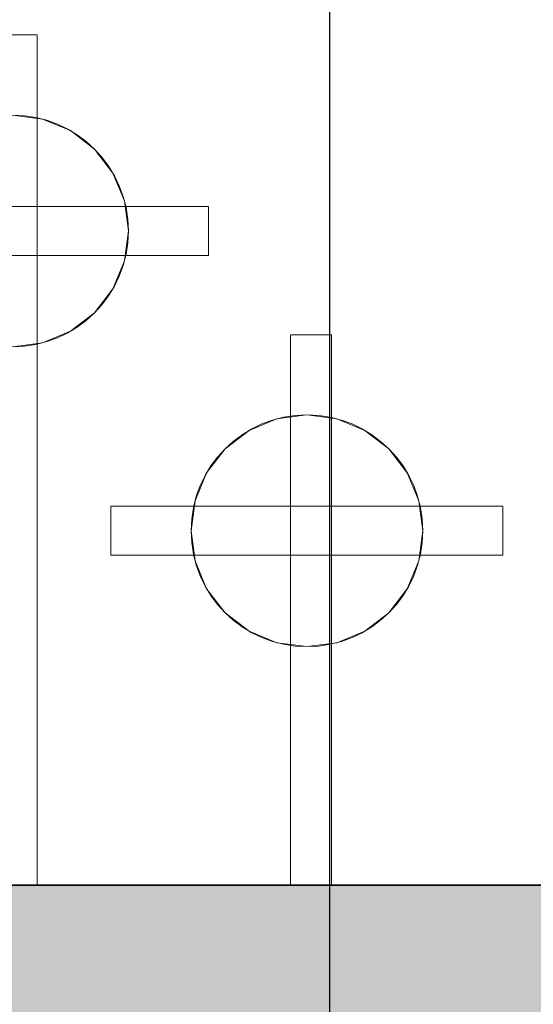
# Model space of a CAD drawing. Units: inches. Extents: x 2696 to 3240, y 1564 to 2310.
# Tile 31 of 76: x 3146.244 to 3150.171, y 1698.791 to 1706.319. Entities that reach past the tile are written whole.
import ezdxf

# ---------------------------------------------------------------- set-up
doc = ezdxf.new("R2010")
doc.units = ezdxf.units.IN
for name, color, linetype, lineweight in [('A-ANNO-DIMS', 3, 'Continuous', 18), ('A-FLOR-FIXT', 8, 'Continuous', 18), ('A-FURN', 251, 'Continuous', 13), ('A-WALL', 7, 'Continuous', 35), ('A-WALL-PATT', 9, 'Continuous', 13)]:
    doc.layers.add(name, color=color, linetype=linetype, lineweight=lineweight)
doc.layers.add('FURNITURE', color=250, linetype='Continuous')
doc.styles.add('TIMES NEW', font='times.ttf')
doc.dimstyles.new('Siddhuu', dxfattribs={"dimtxt": 6, "dimasz": 2.5, "dimexe": 1.25, "dimexo": 0.625, "dimtad": 1, "dimdec": 1, "dimlunit": 4, "dimtxsty": 'TIMES NEW', "dimcen": 2.5, "dimclrd": 256, "dimclre": 1, "dimclrt": 7, "dimadec": 0, "dimazin": 0, "dimtfac": 1, "dimtdec": 1, "dimtmove": 0, "dimatfit": 3, "dimfxl": 1, "dimtolj": 1, "dimlwd": -1, "dimarcsym": 0})

# ---------------------------------------------------------------- blocks, each defined once
blk = doc.blocks.new('A$C1af1f523')
at = {"layer": 'A-FURN'}
for p, q in [((-5.1906, 1.6871), (-5.1901, -1.3115)), ((-5.1906, 1.6871, 0.5), (-5.1901, -1.3115, 0.5)), ((-4.8156, 1.6871), (-4.8151, -1.3115)), ((-4.8156, 1.6871, 0.5), (-4.8151, -1.3115, 0.5)), ((-6.5015, 0.3114), (-6.5015, 0)), ((-6.5015, 0.3114, 0.5), (-6.5015, 0, 0.5)), ((0, 0), (-6.5015, 0)), ((0, 0, 0.5), (-6.5015, 0, 0.5)), ((-6.5015, 0), (-6.5015, 0, 0.5)), ((-6.5015, 0), (-6.5015, -0.0011)), ((-6.5015, 0, 0.5), (-6.5015, -0.0011, 0.5)), ((-6.5015, -0.0011), (-6.5015, -0.0011, 0.5)), ((-5.8585, -0.0418), (-5.8585, -0.0418, 0.5)), ((-4.1468, -0.0418), (-4.1468, -0.0418, 0.5)), ((-5.77, -0.2555), (-5.77, -0.2555, 0.5)), ((-4.2353, -0.2555), (-4.2353, -0.2555, 0.5)), ((-5.6292, -0.439), (-5.6292, -0.439, 0.5)), ((-4.3761, -0.439), (-4.3761, -0.439, 0.5)), ((-5.4457, -0.5798), (-5.4457, -0.5798, 0.5)), ((-4.5596, -0.5798), (-4.5596, -0.5798, 0.5)), ((-2.898, -0.5642), (-2.898, -3.5628)), ((-2.898, -0.5642, 0.5), (-2.898, -3.5628, 0.5)), ((-2.898, -0.5642), (-2.898, -0.5642, 0.5)), ((-2.523, -0.5642), (-2.898, -0.5642)), ((-2.523, -0.5642, 0.5), (-2.898, -0.5642, 0.5)), ((-2.523, -0.5642), (-2.523, -3.5628)), ((-2.523, -0.5642, 0.5), (-2.523, -3.5628, 0.5)), ((-2.523, -0.5642), (-2.523, -0.5642, 0.5)), ((-5.232, -0.6683), (-5.232, -0.6683, 0.5)), ((-4.7733, -0.6683), (-4.7733, -0.6683, 0.5)), ((-5.0026, -0.6985), (-5.0026, -0.6985, 0.5)), ((-2.7105, -1.1778), (-2.7105, -1.1778, 0.5)), ((-2.9398, -1.208), (-2.9398, -1.208, 0.5)), ((-2.4812, -1.208), (-2.4812, -1.208, 0.5)), ((-5.1901, -1.3115), (-5.1901, -1.3115, 0.5)), ((-4.8151, -1.3115), (-5.1878, -1.3115)), ((-4.8151, -1.3115, 0.5), (-5.1878, -1.3115, 0.5)), ((-5.1878, -1.3115), (-5.1878, -1.3115, 0.5)), ((-4.8151, -1.3115), (-4.8151, -1.3115, 0.5)), ((-3.1535, -1.2965), (-3.1535, -1.2965, 0.5)), ((-2.2675, -1.2965), (-2.2675, -1.2965, 0.5)), ((-3.337, -1.4373), (-3.337, -1.4373, 0.5)), ((-2.084, -1.4373), (-2.084, -1.4373, 0.5)), ((-3.4778, -1.6208), (-3.4778, -1.6208, 0.5)), ((-1.9432, -1.6208), (-1.9432, -1.6208, 0.5)), ((-3.5664, -1.8345), (-3.5664, -1.8345, 0.5)), ((-1.8547, -1.8345), (-1.8547, -1.8345, 0.5)), ((0, -1.9388), (-4.2094, -1.9388)), ((0, -1.9388, 0.5), (-4.2094, -1.9388, 0.5)), ((-4.2094, -1.9388), (-4.2094, -1.9388, 0.5)), ((-4.2094, -1.9399), (-4.2094, -2.2513)), ((-4.2094, -1.9399, 0.5), (-4.2094, -2.2513, 0.5)), ((-4.2094, -1.9399), (-4.2094, -1.9399, 0.5)), ((-3.5965, -2.0638), (-3.5965, -2.0638, 0.5)), ((-1.8245, -2.0638), (-1.8245, -2.0638, 0.5)), ((0, -2.2513), (-4.2094, -2.2513)), ((0, -2.2513, 0.5), (-4.2094, -2.2513, 0.5)), ((-4.2094, -2.2513), (-4.2094, -2.2513, 0.5)), ((-4.2094, -2.2513), (-4.2094, -2.2524)), ((-4.2094, -2.2513, 0.5), (-4.2094, -2.2524, 0.5)), ((-4.2094, -2.2524), (-4.2094, -2.2524, 0.5)), ((-3.5664, -2.2931), (-3.5664, -2.2931, 0.5)), ((-1.8547, -2.2931), (-1.8547, -2.2931, 0.5)), ((-3.4778, -2.5068), (-3.4778, -2.5068, 0.5)), ((-1.9432, -2.5068), (-1.9432, -2.5068, 0.5)), ((-3.337, -2.6903), (-3.337, -2.6903, 0.5)), ((-2.084, -2.6903), (-2.084, -2.6903, 0.5)), ((-3.1535, -2.8311), (-3.1535, -2.8311, 0.5)), ((-2.2675, -2.8311), (-2.2675, -2.8311, 0.5)), ((-2.9398, -2.9196), (-2.9398, -2.9196, 0.5)), ((-2.4812, -2.9196), (-2.4812, -2.9196, 0.5)), ((-2.7105, -2.9498), (-2.7105, -2.9498, 0.5)), ((-2.898, -3.5628), (-2.898, -3.5628, 0.5)), ((-2.523, -3.5628), (-2.8956, -3.5628)), ((-2.523, -3.5628, 0.5), (-2.8956, -3.5628, 0.5)), ((-2.8956, -3.5628), (-2.8956, -3.5628, 0.5)), ((-2.523, -3.5628), (-2.523, -3.5628, 0.5))]:
    blk.add_line(p, q, dxfattribs=at)
for centre in [(-5.0026, 0.1875), (-5.0026, 0.1875, 0.5), (-2.7105, -2.0638), (-2.7105, -2.0638, 0.5)]:
    blk.add_circle(centre, 0.886, dxfattribs=at)
at = {"layer": 'FURNITURE'}
for p, q in [((0, 0), (0, 0, 0.5)), ((0, -1.9388), (0, -1.9388, 0.5)), ((0, -2.2513), (0, -2.2513, 0.5))]:
    blk.add_line(p, q, dxfattribs=at)
at = {"layer": 'A-FURN'}
mesh = blk.add_polyface(dxfattribs=at)
corners = [(-5.1901, -1.3115, 0.5), (-5.1906, 1.6871), (-5.1901, -1.3115), (-5.1906, 1.6871, 0.5)]
mesh.append_faces([[corners[k] for k in face] for face in [(2, 1, 0), (3, 0, 1)]], dxfattribs={"vtx1": -1})
mesh = blk.add_polyface(dxfattribs=at)
corners = [(-4.8151, -1.3115, 0.5), (-4.8156, 1.6871), (-4.8151, -1.3115), (-4.8156, 1.6871, 0.5)]
mesh.append_faces([[corners[k] for k in face] for face in [(2, 1, 0), (3, 0, 1)]], dxfattribs={"vtx1": -1})
mesh = blk.add_polyface(dxfattribs=at)
corners = [(-6.5015, -0.0011, 0.5), (-6.5015, 0), (-6.5015, -0.0011), (-6.5015, 0.3114), (-6.5015, 0.3114, 0.5), (-6.5015, 0, 0.5)]
mesh.append_faces([[corners[k] for k in face] for face in [(3, 0, 1), (4, 0, 3)]], dxfattribs={"vtx0": -1, "vtx1": -1})
mesh.append_faces([[corners[k] for k in face] for face in [(2, 1, 0), (5, 0, 4)]], dxfattribs={"vtx1": -1})
mesh = blk.add_polyface(dxfattribs=at)
corners = [(-5.8887, 0.1875, 0.5), (-5.8585, -0.0418), (-5.8887, 0.1875), (-5.8585, -0.0418, 0.5)]
mesh.append_faces([[corners[k] for k in face] for face in [(2, 1, 0), (3, 0, 1)]], dxfattribs={"vtx1": -1})
mesh = blk.add_polyface(dxfattribs=at)
corners = [(-4.1468, -0.0418, 0.5), (-4.1166, 0.1875), (-4.1468, -0.0418), (-4.1166, 0.1875, 0.5)]
mesh.append_faces([[corners[k] for k in face] for face in [(2, 1, 0), (3, 0, 1)]], dxfattribs={"vtx1": -1})
mesh = blk.add_polyface(dxfattribs=at)
corners = [(0, 0, 0.5), (-6.5015, 0), (-6.5015, 0, 0.5), (0, 0)]
mesh.append_faces([[corners[k] for k in face] for face in [(2, 1, 0), (3, 0, 1)]], dxfattribs={"vtx1": -1})
mesh = blk.add_polyface(dxfattribs=at)
corners = [(-5.8585, -0.0418, 0.5), (-5.77, -0.2555), (-5.8585, -0.0418), (-5.77, -0.2555, 0.5)]
mesh.append_faces([[corners[k] for k in face] for face in [(2, 1, 0), (3, 0, 1)]], dxfattribs={"vtx1": -1})
mesh = blk.add_polyface(dxfattribs=at)
corners = [(-4.2353, -0.2555, 0.5), (-4.1468, -0.0418), (-4.2353, -0.2555), (-4.1468, -0.0418, 0.5)]
mesh.append_faces([[corners[k] for k in face] for face in [(2, 1, 0), (3, 0, 1)]], dxfattribs={"vtx1": -1})
mesh = blk.add_polyface(dxfattribs=at)
corners = [(-5.77, -0.2555, 0.5), (-5.6292, -0.439), (-5.77, -0.2555), (-5.6292, -0.439, 0.5)]
mesh.append_faces([[corners[k] for k in face] for face in [(2, 1, 0), (3, 0, 1)]], dxfattribs={"vtx1": -1})
mesh = blk.add_polyface(dxfattribs=at)
corners = [(-4.3761, -0.439, 0.5), (-4.2353, -0.2555), (-4.3761, -0.439), (-4.2353, -0.2555, 0.5)]
mesh.append_faces([[corners[k] for k in face] for face in [(2, 1, 0), (3, 0, 1)]], dxfattribs={"vtx1": -1})
mesh = blk.add_polyface(dxfattribs=at)
corners = [(-5.4457, -0.5798, 0.5), (-5.6292, -0.439), (-5.6292, -0.439, 0.5), (-5.4457, -0.5798)]
mesh.append_faces([[corners[k] for k in face] for face in [(2, 1, 0), (3, 0, 1)]], dxfattribs={"vtx1": -1})
mesh = blk.add_polyface(dxfattribs=at)
corners = [(-4.3761, -0.439, 0.5), (-4.5596, -0.5798), (-4.5596, -0.5798, 0.5), (-4.3761, -0.439)]
mesh.append_faces([[corners[k] for k in face] for face in [(2, 1, 0), (3, 0, 1)]], dxfattribs={"vtx1": -1})
mesh = blk.add_polyface(dxfattribs=at)
corners = [(-5.232, -0.6683, 0.5), (-5.4457, -0.5798), (-5.4457, -0.5798, 0.5), (-5.232, -0.6683)]
mesh.append_faces([[corners[k] for k in face] for face in [(2, 1, 0), (3, 0, 1)]], dxfattribs={"vtx1": -1})
mesh = blk.add_polyface(dxfattribs=at)
corners = [(-4.5596, -0.5798, 0.5), (-4.7733, -0.6683), (-4.7733, -0.6683, 0.5), (-4.5596, -0.5798)]
mesh.append_faces([[corners[k] for k in face] for face in [(2, 1, 0), (3, 0, 1)]], dxfattribs={"vtx1": -1})
mesh = blk.add_polyface(dxfattribs=at)
corners = [(-2.898, -3.5628, 0.5), (-2.898, -0.5642), (-2.898, -3.5628), (-2.898, -0.5642, 0.5)]
mesh.append_faces([[corners[k] for k in face] for face in [(2, 1, 0), (3, 0, 1)]], dxfattribs={"vtx1": -1})
mesh = blk.add_polyface(dxfattribs=at)
corners = [(-2.523, -0.5642, 0.5), (-2.898, -0.5642), (-2.898, -0.5642, 0.5), (-2.523, -0.5642)]
mesh.append_faces([[corners[k] for k in face] for face in [(2, 1, 0), (3, 0, 1)]], dxfattribs={"vtx1": -1})
mesh = blk.add_polyface(dxfattribs=at)
corners = [(-2.523, -3.5628, 0.5), (-2.523, -0.5642), (-2.523, -3.5628), (-2.523, -0.5642, 0.5)]
mesh.append_faces([[corners[k] for k in face] for face in [(2, 1, 0), (3, 0, 1)]], dxfattribs={"vtx1": -1})
mesh = blk.add_polyface(dxfattribs=at)
corners = [(-5.0026, -0.6985, 0.5), (-5.232, -0.6683), (-5.232, -0.6683, 0.5), (-5.0026, -0.6985)]
mesh.append_faces([[corners[k] for k in face] for face in [(2, 1, 0), (3, 0, 1)]], dxfattribs={"vtx1": -1})
mesh = blk.add_polyface(dxfattribs=at)
corners = [(-4.7733, -0.6683, 0.5), (-5.0026, -0.6985), (-5.0026, -0.6985, 0.5), (-4.7733, -0.6683)]
mesh.append_faces([[corners[k] for k in face] for face in [(2, 1, 0), (3, 0, 1)]], dxfattribs={"vtx1": -1})
mesh = blk.add_polyface(dxfattribs=at)
corners = [(-2.7105, -1.1778), (-2.9398, -1.208, 0.5), (-2.9398, -1.208), (-2.7105, -1.1778, 0.5)]
mesh.append_faces([[corners[k] for k in face] for face in [(2, 1, 0), (3, 0, 1)]], dxfattribs={"vtx1": -1})
mesh = blk.add_polyface(dxfattribs=at)
corners = [(-2.4812, -1.208), (-2.7105, -1.1778, 0.5), (-2.7105, -1.1778), (-2.4812, -1.208, 0.5)]
mesh.append_faces([[corners[k] for k in face] for face in [(2, 1, 0), (3, 0, 1)]], dxfattribs={"vtx1": -1})
mesh = blk.add_polyface(dxfattribs=at)
corners = [(-2.9398, -1.208), (-3.1535, -1.2965, 0.5), (-3.1535, -1.2965), (-2.9398, -1.208, 0.5)]
mesh.append_faces([[corners[k] for k in face] for face in [(2, 1, 0), (3, 0, 1)]], dxfattribs={"vtx1": -1})
mesh = blk.add_polyface(dxfattribs=at)
corners = [(-2.2675, -1.2965), (-2.4812, -1.208, 0.5), (-2.4812, -1.208), (-2.2675, -1.2965, 0.5)]
mesh.append_faces([[corners[k] for k in face] for face in [(2, 1, 0), (3, 0, 1)]], dxfattribs={"vtx1": -1})
mesh = blk.add_polyface(dxfattribs=at)
corners = [(-4.8151, -1.3115, 0.5), (-5.1878, -1.3115), (-5.1878, -1.3115, 0.5), (-4.8151, -1.3115)]
mesh.append_faces([[corners[k] for k in face] for face in [(2, 1, 0), (3, 0, 1)]], dxfattribs={"vtx1": -1})
mesh = blk.add_polyface(dxfattribs=at)
corners = [(-3.1535, -1.2965), (-3.337, -1.4373, 0.5), (-3.337, -1.4373), (-3.1535, -1.2965, 0.5)]
mesh.append_faces([[corners[k] for k in face] for face in [(2, 1, 0), (3, 0, 1)]], dxfattribs={"vtx1": -1})
mesh = blk.add_polyface(dxfattribs=at)
corners = [(-2.084, -1.4373), (-2.2675, -1.2965, 0.5), (-2.2675, -1.2965), (-2.084, -1.4373, 0.5)]
mesh.append_faces([[corners[k] for k in face] for face in [(2, 1, 0), (3, 0, 1)]], dxfattribs={"vtx1": -1})
mesh = blk.add_polyface(dxfattribs=at)
corners = [(-3.337, -1.4373, 0.5), (-3.4778, -1.6208), (-3.337, -1.4373), (-3.4778, -1.6208, 0.5)]
mesh.append_faces([[corners[k] for k in face] for face in [(2, 1, 0), (3, 0, 1)]], dxfattribs={"vtx1": -1})
mesh = blk.add_polyface(dxfattribs=at)
corners = [(-1.9432, -1.6208, 0.5), (-2.084, -1.4373), (-1.9432, -1.6208), (-2.084, -1.4373, 0.5)]
mesh.append_faces([[corners[k] for k in face] for face in [(2, 1, 0), (3, 0, 1)]], dxfattribs={"vtx1": -1})
mesh = blk.add_polyface(dxfattribs=at)
corners = [(-3.4778, -1.6208, 0.5), (-3.5664, -1.8345), (-3.4778, -1.6208), (-3.5664, -1.8345, 0.5)]
mesh.append_faces([[corners[k] for k in face] for face in [(2, 1, 0), (3, 0, 1)]], dxfattribs={"vtx1": -1})
mesh = blk.add_polyface(dxfattribs=at)
corners = [(-1.8547, -1.8345, 0.5), (-1.9432, -1.6208), (-1.8547, -1.8345), (-1.9432, -1.6208, 0.5)]
mesh.append_faces([[corners[k] for k in face] for face in [(2, 1, 0), (3, 0, 1)]], dxfattribs={"vtx1": -1})
mesh = blk.add_polyface(dxfattribs=at)
corners = [(-3.5664, -1.8345, 0.5), (-3.5965, -2.0638), (-3.5664, -1.8345), (-3.5965, -2.0638, 0.5)]
mesh.append_faces([[corners[k] for k in face] for face in [(2, 1, 0), (3, 0, 1)]], dxfattribs={"vtx1": -1})
mesh = blk.add_polyface(dxfattribs=at)
corners = [(-1.8245, -2.0638, 0.5), (-1.8547, -1.8345), (-1.8245, -2.0638), (-1.8547, -1.8345, 0.5)]
mesh.append_faces([[corners[k] for k in face] for face in [(2, 1, 0), (3, 0, 1)]], dxfattribs={"vtx1": -1})
mesh = blk.add_polyface(dxfattribs=at)
corners = [(0, -1.9388, 0.5), (-4.2094, -1.9388), (-4.2094, -1.9388, 0.5), (0, -1.9388)]
mesh.append_faces([[corners[k] for k in face] for face in [(2, 1, 0), (3, 0, 1)]], dxfattribs={"vtx1": -1})
mesh = blk.add_polyface(dxfattribs=at)
corners = [(-4.2094, -2.2524, 0.5), (-4.2094, -2.2513), (-4.2094, -2.2524), (-4.2094, -1.9399), (-4.2094, -1.9399, 0.5), (-4.2094, -2.2513, 0.5)]
mesh.append_faces([[corners[k] for k in face] for face in [(3, 0, 1), (4, 0, 3)]], dxfattribs={"vtx0": -1, "vtx1": -1})
mesh.append_faces([[corners[k] for k in face] for face in [(2, 1, 0), (5, 0, 4)]], dxfattribs={"vtx1": -1})
mesh = blk.add_polyface(dxfattribs=at)
corners = [(-3.5965, -2.0638, 0.5), (-3.5664, -2.2931), (-3.5965, -2.0638), (-3.5664, -2.2931, 0.5)]
mesh.append_faces([[corners[k] for k in face] for face in [(2, 1, 0), (3, 0, 1)]], dxfattribs={"vtx1": -1})
mesh = blk.add_polyface(dxfattribs=at)
corners = [(-1.8547, -2.2931, 0.5), (-1.8245, -2.0638), (-1.8547, -2.2931), (-1.8245, -2.0638, 0.5)]
mesh.append_faces([[corners[k] for k in face] for face in [(2, 1, 0), (3, 0, 1)]], dxfattribs={"vtx1": -1})
mesh = blk.add_polyface(dxfattribs=at)
corners = [(0, -2.2513, 0.5), (-4.2094, -2.2513), (-4.2094, -2.2513, 0.5), (0, -2.2513)]
mesh.append_faces([[corners[k] for k in face] for face in [(2, 1, 0), (3, 0, 1)]], dxfattribs={"vtx1": -1})
mesh = blk.add_polyface(dxfattribs=at)
corners = [(-3.5664, -2.2931, 0.5), (-3.4778, -2.5068), (-3.5664, -2.2931), (-3.4778, -2.5068, 0.5)]
mesh.append_faces([[corners[k] for k in face] for face in [(2, 1, 0), (3, 0, 1)]], dxfattribs={"vtx1": -1})
mesh = blk.add_polyface(dxfattribs=at)
corners = [(-1.9432, -2.5068, 0.5), (-1.8547, -2.2931), (-1.9432, -2.5068), (-1.8547, -2.2931, 0.5)]
mesh.append_faces([[corners[k] for k in face] for face in [(2, 1, 0), (3, 0, 1)]], dxfattribs={"vtx1": -1})
mesh = blk.add_polyface(dxfattribs=at)
corners = [(-3.4778, -2.5068, 0.5), (-3.337, -2.6903), (-3.4778, -2.5068), (-3.337, -2.6903, 0.5)]
mesh.append_faces([[corners[k] for k in face] for face in [(2, 1, 0), (3, 0, 1)]], dxfattribs={"vtx1": -1})
mesh = blk.add_polyface(dxfattribs=at)
corners = [(-2.084, -2.6903, 0.5), (-1.9432, -2.5068), (-2.084, -2.6903), (-1.9432, -2.5068, 0.5)]
mesh.append_faces([[corners[k] for k in face] for face in [(2, 1, 0), (3, 0, 1)]], dxfattribs={"vtx1": -1})
mesh = blk.add_polyface(dxfattribs=at)
corners = [(-3.1535, -2.8311, 0.5), (-3.337, -2.6903), (-3.337, -2.6903, 0.5), (-3.1535, -2.8311)]
mesh.append_faces([[corners[k] for k in face] for face in [(2, 1, 0), (3, 0, 1)]], dxfattribs={"vtx1": -1})
mesh = blk.add_polyface(dxfattribs=at)
corners = [(-2.084, -2.6903, 0.5), (-2.2675, -2.8311), (-2.2675, -2.8311, 0.5), (-2.084, -2.6903)]
mesh.append_faces([[corners[k] for k in face] for face in [(2, 1, 0), (3, 0, 1)]], dxfattribs={"vtx1": -1})
mesh = blk.add_polyface(dxfattribs=at)
corners = [(-2.9398, -2.9196, 0.5), (-3.1535, -2.8311), (-3.1535, -2.8311, 0.5), (-2.9398, -2.9196)]
mesh.append_faces([[corners[k] for k in face] for face in [(2, 1, 0), (3, 0, 1)]], dxfattribs={"vtx1": -1})
mesh = blk.add_polyface(dxfattribs=at)
corners = [(-2.2675, -2.8311, 0.5), (-2.4812, -2.9196), (-2.4812, -2.9196, 0.5), (-2.2675, -2.8311)]
mesh.append_faces([[corners[k] for k in face] for face in [(2, 1, 0), (3, 0, 1)]], dxfattribs={"vtx1": -1})
mesh = blk.add_polyface(dxfattribs=at)
corners = [(-2.7105, -2.9498, 0.5), (-2.9398, -2.9196), (-2.9398, -2.9196, 0.5), (-2.7105, -2.9498)]
mesh.append_faces([[corners[k] for k in face] for face in [(2, 1, 0), (3, 0, 1)]], dxfattribs={"vtx1": -1})
mesh = blk.add_polyface(dxfattribs=at)
corners = [(-2.4812, -2.9196, 0.5), (-2.7105, -2.9498), (-2.7105, -2.9498, 0.5), (-2.4812, -2.9196)]
mesh.append_faces([[corners[k] for k in face] for face in [(2, 1, 0), (3, 0, 1)]], dxfattribs={"vtx1": -1})
mesh = blk.add_polyface(dxfattribs=at)
corners = [(-2.523, -3.5628, 0.5), (-2.8956, -3.5628), (-2.8956, -3.5628, 0.5), (-2.523, -3.5628)]
mesh.append_faces([[corners[k] for k in face] for face in [(2, 1, 0), (3, 0, 1)]], dxfattribs={"vtx1": -1})
blk = doc.blocks.new('*D51')
at = {"layer": 'A-ANNO-DIMS', "color": 1, "lineweight": -2, "transparency": 16777216}
for p, q in [((3016.6114, 1979.5761), (3016.6114, 1568.9511)), ((3148.6114, 1979.5761), (3148.6114, 1568.9511))]:
    blk.add_line(p, q, dxfattribs=at)
at = {"layer": 'A-ANNO-DIMS', "transparency": 16777216}
blk.add_line((3019.1114, 1570.2011), (3146.1114, 1570.2011), dxfattribs=at)
for points in [[(3019.1114, 1570.6178), (3019.1114, 1569.7844), (3016.6114, 1570.2011)], [(3146.1114, 1570.6178), (3146.1114, 1569.7844), (3148.6114, 1570.2011)]]:
    blk.add_solid(points, dxfattribs=at)
at = {"layer": 'Defpoints', "color": 0, "transparency": 16777216}
for p in [(3016.6114, 1980.2011), (3148.6114, 1980.2011), (3148.6114, 1570.2011)]:
    blk.add_point(p, dxfattribs=at)
at = {"layer": 'A-ANNO-DIMS', "color": 7, "transparency": 16777216, "insert": (3082.6114, 1573.878), "char_height": 6, "attachment_point": 5, "style": 'TIMES NEW'}
blk.add_mtext('\\A1;11\'-0"', dxfattribs=at)
blk = doc.blocks.new('*D52')
at = {"layer": 'A-ANNO-DIMS', "color": 1, "lineweight": -2, "transparency": 16777216}
for p, q in [((3148.6114, 1979.5761), (3148.6114, 1568.9511)), ((3190.6114, 1979.5761), (3190.6114, 1568.9511))]:
    blk.add_line(p, q, dxfattribs=at)
at = {"layer": 'A-ANNO-DIMS', "transparency": 16777216}
blk.add_line((3151.1114, 1570.2011), (3188.1114, 1570.2011), dxfattribs=at)
for points in [[(3151.1114, 1570.6178), (3151.1114, 1569.7844), (3148.6114, 1570.2011)], [(3188.1114, 1570.6178), (3188.1114, 1569.7844), (3190.6114, 1570.2011)]]:
    blk.add_solid(points, dxfattribs=at)
at = {"layer": 'Defpoints', "color": 0, "transparency": 16777216}
for p in [(3148.6114, 1980.2011), (3190.6114, 1980.2011), (3190.6114, 1570.2011)]:
    blk.add_point(p, dxfattribs=at)
at = {"layer": 'A-ANNO-DIMS', "color": 7, "transparency": 16777216, "insert": (3169.6114, 1573.878), "char_height": 6, "attachment_point": 5, "style": 'TIMES NEW'}
blk.add_mtext('\\A1;3\'-6"', dxfattribs=at)
blk = doc.blocks.new('*D56')
at = {"layer": 'A-ANNO-DIMS', "color": 1, "lineweight": -2, "transparency": 16777216}
for p, q in [((2966.3338, 1884.2011), (3235.8614, 1884.2011)), ((2966.3338, 1665.2011), (3235.8614, 1665.2011))]:
    blk.add_line(p, q, dxfattribs=at)
at = {"layer": 'A-ANNO-DIMS', "transparency": 16777216}
blk.add_line((3234.6114, 1667.7011), (3234.6114, 1881.7011), dxfattribs=at)
for points in [[(3234.1947, 1881.7011), (3235.0281, 1881.7011), (3234.6114, 1884.2011)], [(3234.1947, 1667.7011), (3235.0281, 1667.7011), (3234.6114, 1665.2011)]]:
    blk.add_solid(points, dxfattribs=at)
at = {"layer": 'Defpoints', "color": 0, "transparency": 16777216}
for p in [(2965.7088, 1884.2011), (3234.6114, 1884.2011), (2965.7088, 1665.2011)]:
    blk.add_point(p, dxfattribs=at)
at = {"layer": 'A-ANNO-DIMS', "color": 7, "transparency": 16777216, "insert": (3230.9345, 1774.7011), "char_height": 6, "attachment_point": 5, "rotation": 90, "style": 'TIMES NEW'}
blk.add_mtext('\\A1;18\'-3"', dxfattribs=at)

msp = doc.modelspace()

# ---------------------------------------------------------------- hatches: boundary and pattern name
at = {"layer": 'A-WALL-PATT', "transparency": 33554556}
h = msp.add_hatch(color=256, dxfattribs=at)
h.dxf.hatch_style = 1
h.paths.add_polyline_path([(2879.1114, 2253.2011), (2905.9101, 2253.2011), (2905.9101, 2262.2011), (2841.889, 2262.2011), (2841.889, 2253.2011), (2870.1114, 2253.2011), (2870.1114, 2176.6011), (2965.7088, 2176.6011), (2965.7088, 2206.7011), (2973.5828, 2206.7011), (2973.5828, 2215.7011), (2965.7088, 2215.7011), (2965.7088, 2262.2011), (2929.9101, 2262.2011), (2929.9101, 2253.2011), (2956.7088, 2253.2011), (2956.7088, 2185.6011), (2879.1114, 2185.6011)])
h.paths.add_polyline_path([(2782.8338, 2262.2011), (2745.6114, 2262.2011), (2745.6114, 2228.7287), (2754.6114, 2228.7287), (2754.6114, 2253.2011), (2782.8338, 2253.2011)])
h.paths.add_polyline_path([(2754.6114, 2136.2011), (2965.7088, 2136.2011), (2965.7088, 2145.2011), (2879.1114, 2145.2011), (2879.1114, 2147.0735), (2877.3397, 2147.0735), (2870.1114, 2147.0735), (2870.1114, 2145.2011), (2754.6114, 2145.2011), (2754.6114, 2169.6735), (2745.6114, 2169.6735), (2745.6114, 2000.2011), (2754.6114, 2000.2011), (2754.6114, 2019.2011), (2849.0828, 2019.2011), (2849.0828, 2023.7011), (2841.2088, 2023.7011), (2841.2088, 2051.8271), (2836.7088, 2051.8271), (2836.7088, 2023.7011), (2754.6114, 2023.7011), (2754.6114, 2091.2011), (2836.7088, 2091.2011), (2836.7088, 2087.8271), (2841.2088, 2087.8271), (2841.2088, 2095.7011), (2754.6114, 2095.7011)])
h.paths.add_polyline_path([(2965.7088, 2136.2011), (2956.7088, 2136.2011), (2956.7088, 2023.7011), (2885.0828, 2023.7011), (2885.0828, 2019.2011), (2956.7088, 2019.2011), (2956.7088, 1950.5751), (2965.7088, 1950.5751), (2965.7088, 1980.2011), (2973.5828, 1980.2011), (2973.5828, 1989.2011), (2965.7088, 1989.2011)])
h.paths.add_polyline_path([(2754.6114, 1906.7011), (2880.2088, 1906.7011), (2884.7088, 1906.7011), (2956.7088, 1906.7011), (2956.7088, 1792.7011), (2944.7088, 1792.7011), (2944.7088, 1783.7011), (2956.7088, 1783.7011), (2956.7088, 1740.2011), (2884.7088, 1740.2011), (2884.7088, 1783.7011), (2896.7088, 1783.7011), (2896.7088, 1792.7011), (2884.7088, 1792.7011), (2884.7088, 1846.7011), (2880.2088, 1846.7011), (2880.2088, 1740.2011), (2754.6114, 1740.2011), (2754.6114, 1777.2011), (2745.6114, 1777.2011), (2745.6114, 1692.7011), (2754.6114, 1692.7011), (2754.6114, 1731.2011), (2956.7088, 1731.2011), (2956.7088, 1723.3271), (2965.7088, 1723.3271), (2965.7088, 1884.2011), (2973.5828, 1884.2011), (2973.5828, 1893.2011), (2965.7088, 1893.2011), (2965.7088, 1914.5751), (2956.7088, 1914.5751), (2956.7088, 1911.2011), (2754.6114, 1911.2011), (2754.6114, 1930.2011), (2745.6114, 1930.2011), (2745.6114, 1817.2011), (2754.6114, 1817.2011), (2754.6114, 1854.2011), (2826.6114, 1854.2011), (2826.6114, 1868.8271), (2822.1114, 1868.8271), (2822.1114, 1858.7011), (2754.6114, 1858.7011)])
h.paths.add_polyline_path([(2965.7088, 1656.2011), (3008.2374, 1656.2011), (3008.2374, 1665.2011), (2965.7088, 1665.2011), (2965.7088, 1693.3271), (2956.7088, 1693.3271), (2956.7088, 1686.2011), (2934.5828, 1686.2011), (2934.5828, 1681.7011), (2956.7088, 1681.7011), (2956.7088, 1614.2011), (2896.7088, 1614.2011), (2896.7088, 1681.7011), (2904.5828, 1681.7011), (2904.5828, 1686.2011), (2892.2088, 1686.2011), (2892.2088, 1614.2011), (2858.4101, 1614.2011), (2858.4101, 1605.2011), (2965.7088, 1605.2011)])
h.paths.add_polyline_path([(2788.4101, 1614.2011), (2754.6114, 1614.2011), (2754.6114, 1652.7011), (2745.6114, 1652.7011), (2745.6114, 1605.2011), (2788.4101, 1605.2011)])
h.paths.add_polyline_path([(3199.6114, 1633.0476), (3190.6114, 1633.0476), (3190.6114, 1614.2011), (3082.6114, 1614.2011), (3082.6114, 1665.2011), (3070.2374, 1665.2011), (3070.2374, 1656.2011), (3078.1114, 1656.2011), (3078.1114, 1605.2011), (3199.6114, 1605.2011)])
h.paths.add_polyline_path([(3199.6114, 1702.0476), (3190.6114, 1702.0476), (3190.6114, 1699.7011), (3106.6114, 1699.7011), (3106.6114, 1747.7011), (3190.6114, 1747.7011), (3190.6114, 1752.2011), (3082.6114, 1752.2011), (3082.6114, 1760.0751), (3078.1114, 1760.0751), (3078.1114, 1747.7011), (3102.1114, 1747.7011), (3102.1114, 1699.7011), (3078.1114, 1699.7011), (3078.1114, 1695.2011), (3190.6114, 1695.2011), (3190.6114, 1676.3546), (3199.6114, 1676.3546)])
h.paths.add_polyline_path([(3199.6114, 1783.2011), (3190.6114, 1783.2011), (3190.6114, 1745.3546), (3199.6114, 1745.3546)])
h.paths.add_polyline_path([(3082.6114, 1884.2011), (3190.6114, 1884.2011), (3190.6114, 1853.2011), (3199.6114, 1853.2011), (3199.6114, 1901.7011), (3190.6114, 1901.7011), (3190.6114, 1893.2011), (3005.5828, 1893.2011), (3005.5828, 1891.2811), (3005.5828, 1884.2011), (3078.1114, 1884.2011), (3078.1114, 1792.0751), (3082.6114, 1792.0751)])
h.paths.add_polyline_path([(3199.6114, 1994.7011), (3190.6114, 1994.7011), (3190.6114, 1989.2011), (3073.7088, 1989.2011), (3073.7088, 2034.2011), (3069.2088, 2034.2011), (3069.2088, 1989.2011), (3005.5828, 1989.2011), (3005.5828, 1980.2011), (3190.6114, 1980.2011), (3190.6114, 1971.7011), (3199.6114, 1971.7011)])
h.paths.add_polyline_path([(3199.6114, 2155.2011), (3190.6114, 2155.2011), (3190.6114, 2064.7011), (3199.6114, 2064.7011)])
h.paths.add_polyline_path([(3190.6114, 2074.7011), (3106.6114, 2074.7011), (3106.6114, 2122.7011), (3190.6114, 2122.7011), (3190.6114, 2127.2011), (3082.7088, 2127.2011), (3082.7088, 2135.0751), (3073.7088, 2135.0751), (3073.7088, 2122.7011), (3102.1114, 2122.7011), (3102.1114, 2074.7011), (3069.2088, 2074.7011), (3069.2088, 2070.2011), (3190.6114, 2070.2011)])
h.paths.add_polyline_path([(3082.7088, 2253.2011), (3190.6114, 2253.2011), (3190.6114, 2225.2011), (3199.6114, 2225.2011), (3199.6114, 2262.2011), (3073.7088, 2262.2011), (3073.7088, 2215.7011), (3035.5828, 2215.7011), (3035.5828, 2206.7011), (3073.7088, 2206.7011), (3073.7088, 2171.0751), (3082.7088, 2171.0751)])

# ---------------------------------------------------------------- linework, layer by layer
at = {"layer": 'A-WALL'}
msp.add_line((3106.6114, 1699.7011), (3190.6114, 1699.7011), dxfattribs=at)

# ---------------------------------------------------------------- block references
at = {"layer": 'A-FLOR-FIXT', "xscale": -1, "rotation": 90}
msp.add_blockref('A$C1af1f523', (3146.3764, 1699.7011), dxfattribs=at)

# ---------------------------------------------------------------- dimensions: what is measured, and where the dimension line sits
at = {"layer": 'A-ANNO-DIMS'}
for base, p1, p2, picture, middle in [((3148.6114, 1570.2011), (3016.6114, 1980.2011), (3148.6114, 1980.2011), '*D51', (3082.6114, 1573.878)), ((3190.6114, 1570.2011), (3148.6114, 1980.2011), (3190.6114, 1980.2011), '*D52', (3169.6114, 1573.878))]:
    dim = msp.add_linear_dim(base=base, p1=p1, p2=p2, dimstyle='Siddhuu', override={"dimdec": 1, "dimlfac": 1, "dimrnd": 0, "dimzin": 1, "dimdsep": 46, "dimlunit": 4, "dimfrac": 2}, dxfattribs=at)
    dim.commit()
    dim.dimension.update_dxf_attribs({"geometry": picture, "text_midpoint": middle})
dim = msp.add_linear_dim(base=(3234.6114, 1884.2011), p1=(2965.7088, 1665.2011), p2=(2965.7088, 1884.2011), angle=90, dimstyle='Siddhuu', override={"dimdec": 1, "dimlfac": 1, "dimrnd": 0, "dimzin": 1, "dimdsep": 46, "dimlunit": 4, "dimfrac": 2}, dxfattribs=at)
dim.commit()
dim.dimension.update_dxf_attribs({"geometry": '*D56', "text_midpoint": (3230.9345, 1774.7011)})

doc.saveas('drawing.dxf')
